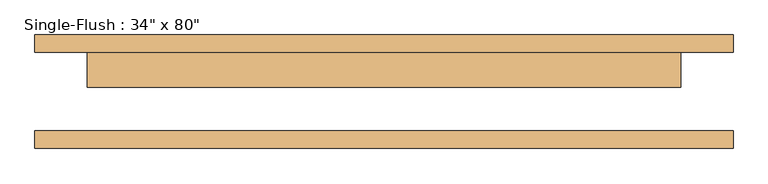
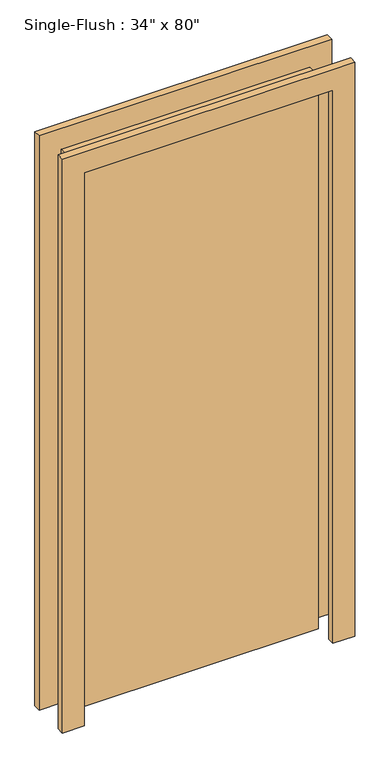
"""IFC4 building model written with IfcOpenShell, lengths in millimetres: door geometry."""

from ifc_helpers import new_model, si_unit, frame, origin, origin_with_axes, place, context, project, spatial, polyline, outline, extrude, source, transform, mapped, element, save


def door_c29894e6(model_context):
    return source(origin(), model_context, "Body", "SweptSolid", [
        extrude(outline(polyline([(2108.2, -508.0), (0.0, -508.0), (0.0, -431.8), (2032.0, -431.8), (2032.0, 431.8), (0.0, 431.8), (0.0, 508.0), (2108.2, 508.0), (2108.2, -508.0)])), frame((0.0, 57.15, 0.0), z_axis=(0.0, 1.0, 0.0), x_axis=(0.0, 0.0, 1.0)), (0.0, 0.0, 1.0), 25.4),
        extrude(outline(polyline([(2108.2, 508.0), (2108.2, -508.0), (0.0, -508.0), (0.0, -431.8), (2032.0, -431.8), (2032.0, 431.8), (0.0, 431.8), (0.0, 508.0), (2108.2, 508.0)])), frame((0.0, -82.55, 0.0), z_axis=(0.0, 1.0, 0.0), x_axis=(0.0, 0.0, 1.0)), (0.0, 0.0, 1.0), 25.4),
        extrude(outline(polyline([(431.8, 6.35), (-431.8, 6.35), (-431.8, 57.15), (431.8, 57.15), (431.8, 6.35)])), origin_with_axes(), (0.0, 0.0, 1.0), 2032.0),
    ])


if __name__ == "__main__":
    model = new_model("IFC4")
    model_context = context("Model", 3, world=origin())
    ifc_project = project(units=[si_unit("LENGTHUNIT", "METRE", prefix="MILLI")], contexts=[model_context])
    site = spatial("IfcSite", under=ifc_project)
    building = spatial("IfcBuilding", under=site)
    placement = place(None, origin())
    door_shape = door_c29894e6(model_context)
    element("IfcDoor", 1, ObjectType="Single-Flush : 34\" x 80\"", at=placement, inside=building, context=model_context, shape_type="MappedRepresentation", body=[
        mapped(door_shape, transform((0.0, 0.0, 0.0), x_axis=(1.0, 0.0, 0.0), y_axis=(0.0, 1.0, 0.0), z_axis=(0.0, 0.0, 1.0))),
    ])
    save(model, "model.ifc")

# Revit data of these elements
# Type "Single-Flush : 34\" x 80\""
#   Type Mark = "7"
#   Construction Type Id = "MDOOR"
#   Assembly Code = "C1020"
#   Analytic Construction = "Metal"
#   Thickness = 0' - 2"
#   Heat Transfer Coefficient (U) = 0.651978 BTU/(h·ft²·°F)
#   Height = 6' - 8"
#   Trim Projection Ext = 0' - 1"
#   Trim Projection Int = 0' - 1"
#   Trim Width = 0' - 3"
#   Width = 2' - 10"
#   Define Thermal Properties by = 1
#   Define Thermal Properties by = 1
#   Door Material = Door - Panel
#   Frame Material = Door - Frame
#   Visual Light Transmittance = 0
#   Solar Heat Gain Coefficient = 0
#   Function = (empty or 0)
#   Wall Closure = (empty or 0)
# Element 1 (IfcDoor, "Single-Flush : 34\" x 80\"")
#   Materials on its faces: "Door - Frame", "Door - Panel"
# Materials
#   "Door - Panel": class "Wood", colour RGB 210 159 95, transparency 0, Cost = 0
#   "Door - Frame": colour RGB 118 70 51, transparency 0, Cost = 0
